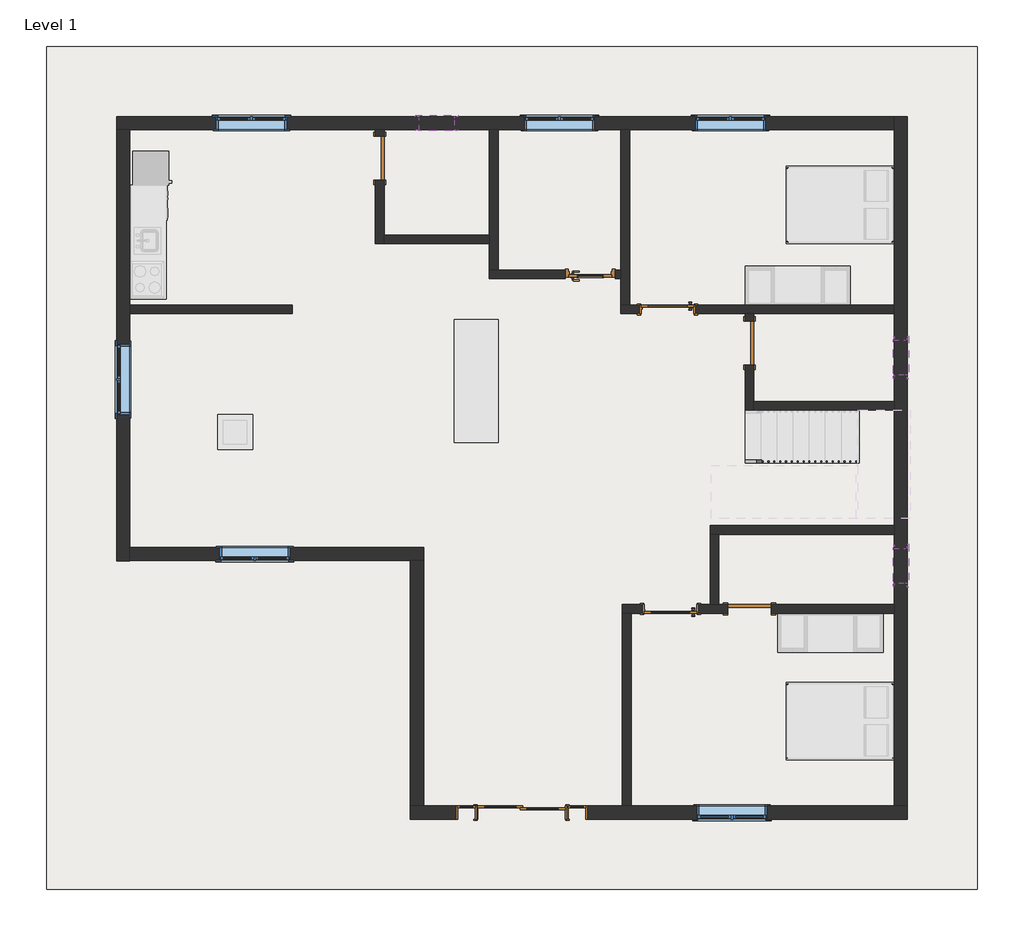
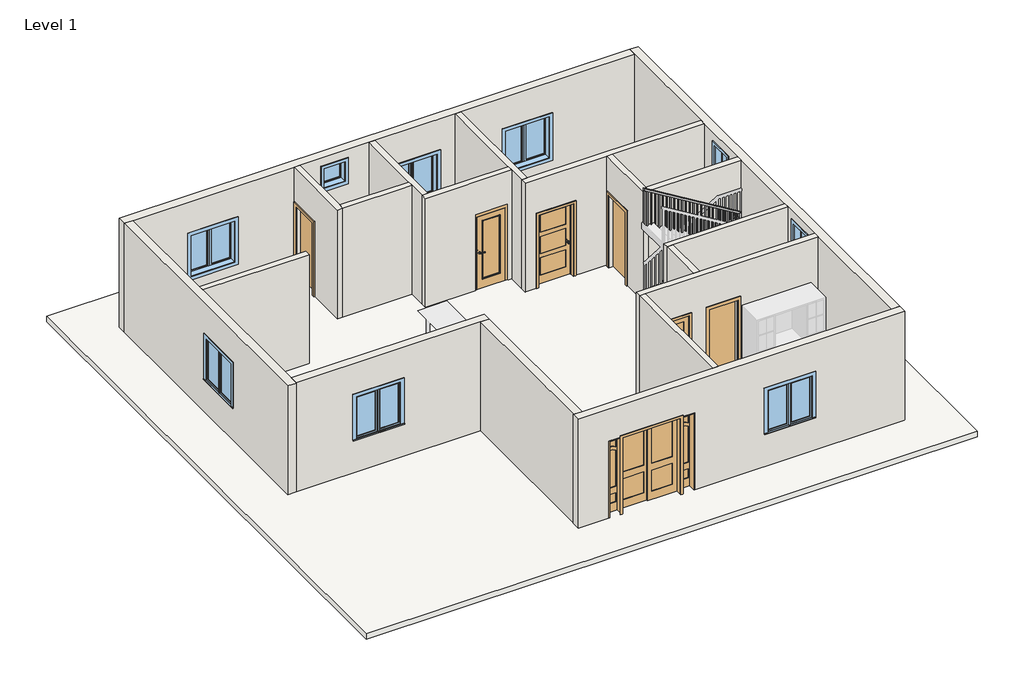
# One storey, part 1 of 2: 19 walls, 9 doors, 9 windows, 1 railing, 1 slab.
# Revit data of these elements (continued)
# Element 6 (IfcDoor, "Door-Passage-Single-Full_Lite : 30\" x 80\"") (continued)
#   Rough Height = 7' - 0"
#   Masonry Inset = 0' - 1"
#   MF Opening Width = 0' - 4"
#   MF Opening Height = 0' - 4"
#   Inset Calculate = 0' - 4"
#   Masonry Frame = yes
#   Dry Wall Frame = no
#   Phase Created = New Construction
#   Materials on its faces: "Metal - Paint Finish - Grey", "Aluminum", "Wood - Birch", "Glass"
# Elements 7, 8, 9 (IfcDoor, "Door-Single-Panel : 30\" x 80\"")
#   Swing Angle = 90.00°
#   Phase Created = New Construction
#   Materials on its faces: "Paint - Sienna", "Wood - Birch - Solid Stained Light Low Gloss"
# Element 10 (IfcRailing, "Handrail - Rectangular")
#   Phase Created = New Construction
# Element 11 (IfcSlab, "Generic - 6\" 2")
#   Height Offset From Level = 0' - 0"
#   Phase Created = New Construction
#   Materials on its faces: "Default Floor"
# Elements 12, 13, 14, 15, 16, 17, 18, 19, 20, 21, 22, 23, 24 (IfcWall, "Generic - 6\"")
#   Top Offset = 0' - 0"
#   Base Offset = 0' - 0"
#   Unconnected Height = 10' - 0"
#   wall height = 10' - 0"
#   Phase Created = New Construction
#   Base Constraint = Level 1
#   Materials on its faces: "Default Wall"
# Elements 25, 26, 27, 28, 29, 30 (IfcWall, "Generic - 9\" 2")
#   Top Offset = 0' - 0"
#   Base Offset = 0' - 0"
#   Unconnected Height = 10' - 0"
#   wall height = 10' - 0"
#   Phase Created = New Construction
#   Base Constraint = Level 1
#   Materials on its faces: "Default Wall"
# Element 31 (IfcWindow, "Casement Dbl with Trim : 48\" x 48\"")
#   Mark = "1"
#   Phase Created = New Construction
#   Materials on its faces: "Sash", "Trim", "Glass"
# Element 32 (IfcWindow, "Casement Dbl with Trim : 48\" x 48\"")
#   Mark = "2"
#   Phase Created = New Construction
#   Materials on its faces: "Sash", "Trim", "Glass"
# Element 33 (IfcWindow, "Casement Dbl with Trim : 48\" x 48\"")
#   Mark = "3"
#   Phase Created = New Construction
#   Materials on its faces: "Sash", "Trim", "Glass"
# Element 34 (IfcWindow, "Casement Dbl with Trim : 48\" x 48\"")
#   Mark = "4"
#   Phase Created = New Construction
#   Materials on its faces: "Sash", "Trim", "Glass"
# Element 35 (IfcWindow, "Casement Dbl with Trim : 48\" x 48\"")
#   Mark = "5"
#   Phase Created = New Construction
#   Materials on its faces: "Sash", "Trim", "Glass"
# Element 36 (IfcWindow, "Casement Dbl with Trim : 48\" x 48\"")
#   Mark = "6"
#   Phase Created = New Construction
#   Materials on its faces: "Sash", "Trim", "Glass"
# Element 37 (IfcWindow, "Transom with Trim : 24\" x 24\"")
#   Mark = "7"
#   Phase Created = New Construction
#   Materials on its faces: "Sash", "Trim", "Glass"
# Element 38 (IfcWindow, "Transom with Trim : 24\" x 24\"")
#   Mark = "8"
#   Phase Created = New Construction
#   Materials on its faces: "Sash", "Trim", "Glass"
# Element 39 (IfcWindow, "Transom with Trim : 24\" x 24\"")
#   Mark = "9"
#   Phase Created = New Construction
#   Materials on its faces: "Sash", "Trim", "Glass"
# Materials
#   "Cherry": class "Wood", colour RGB 226 177 128, transparency 0, Description = "Prunus Serotina", Cost = 0
#   "Glass": class "Glass", colour RGB 0 128 192, transparency 0.75, Description = "Soda Lime Glass", Cost = 0
#   "Aluminum": class "Metal", colour RGB 247 247 247, transparency 0, Description = "Aluminum 6061", Cost = 0
#   "Wood - Birch": class "Wood", colour RGB 166 116 52, transparency 0, Cost = 0
#   "Metal - Paint Finish - Grey": class "Paint", colour RGB 104 104 104, transparency 0, Cost = 0
#   "Wood - Birch - Solid Stained Light Low Gloss": class "Wood", colour RGB 210 159 95, transparency 0, Cost = 0
#   "Paint - Sienna": colour RGB 118 70 51, transparency 0, Cost = 0
#   "Sash": class "Wood", colour RGB 224 178 126, transparency 0
#   "Trim": class "Wood", colour RGB 224 178 126, transparency 0
#   "Default Floor": colour RGB 128 128 128, transparency 0
#   "Default Wall": colour RGB 128 128 128, transparency 0
